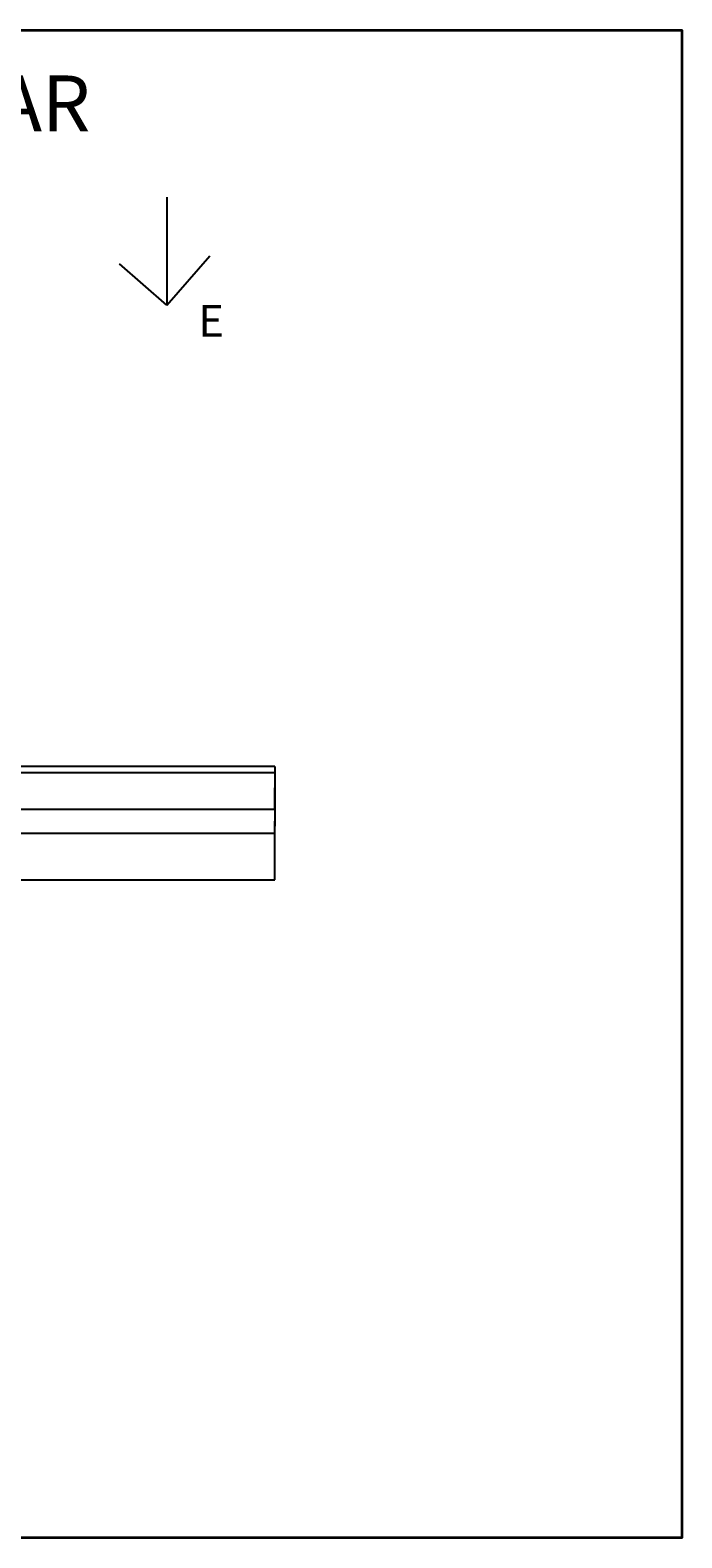
# Model space of a CAD drawing. Units: millimetres. Extents: x -5297 to 19051, y -14478 to 4427.
# Tile 4 of 4: x 10888 to 19051, y -14478 to 4427. Entities that reach past the tile are written whole.
import ezdxf

# ---------------------------------------------------------------- set-up
doc = ezdxf.new("R2010")
doc.units = ezdxf.units.MM
for name, color, linetype, lineweight in [('A-ANNO-DIMS', 2, 'Continuous', 18), ('A-ANNO-SYMB', 7, 'Continuous', 25), ('A-ANNO-TTLB', 7, 'Continuous', 35)]:
    doc.layers.add(name, color=color, linetype=linetype, lineweight=lineweight)
doc.styles.get("Standard").update_dxf_attribs({"font": 'arial.ttf'})
doc.dimstyles.get("Standard").update_dxf_attribs({"dimtxt": 0.18, "dimasz": 0.18, "dimexe": 0.18, "dimexo": 0.0625, "dimgap": 0.09, "dimtad": 0, "dimtih": 1, "dimtoh": 1, "dimdec": 4, "dimzin": 0, "dimdsep": 46, "dimtxsty": 'Standard', "dimcen": 0.09, "dimadec": 0, "dimazin": 0, "dimtfac": 1, "dimtdec": 4, "dimtofl": 0, "dimtmove": 0, "dimatfit": 3, "dimfxl": 1, "dimtolj": 1, "dimtzin": 0, "dimarcsym": 0})

# ---------------------------------------------------------------- blocks, each defined once
blk = doc.blocks.new('*D32')
at = {"layer": 'A-ANNO-DIMS', "color": 0, "lineweight": -2, "transparency": 16777216}
for p, q in [((8901.231442000004, -4880.010677000002), (13950.79322200001, -4880.010677000001)), ((13950.61322200001, -4880.190677000001), (13950.61322200001, -5553.628712470669)), ((13950.61322200001, -6227.430677000002), (13950.61322200001, -5553.992641529333)), ((8901.231442000004, -6227.610677000003), (13950.79322200001, -6227.610677000003))]:
    blk.add_line(p, q, dxfattribs=at)
at = {"layer": 'A-ANNO-DIMS', "color": 0, "transparency": 16777216}
for points in [[(13950.58322200001, -4880.190677000001), (13950.64322200001, -4880.190677000001), (13950.61322200001, -4880.010677000001)], [(13950.58322200001, -6227.430677000002), (13950.64322200001, -6227.430677000002), (13950.61322200001, -6227.610677000003)]]:
    blk.add_solid(points, dxfattribs=at)
at = {"layer": 'Defpoints', "color": 0, "transparency": 16777216}
for p in [(8901.168942000004, -4880.010677000002), (13950.61322200001, -4880.010677000001), (8901.168942000004, -6227.610677000003)]:
    blk.add_point(p, dxfattribs=at)
at = {"layer": 'A-ANNO-DIMS', "color": 0, "transparency": 16777216, "insert": (13950.61322200001, -5553.810677000004), "char_height": 0.18, "attachment_point": 5}
blk.add_mtext('\\A1;1347.6', dxfattribs=at)
blk = doc.blocks.new('*D41')
at = {"layer": 'A-ANNO-DIMS', "color": 0, "lineweight": -2, "transparency": 16777216}
for p, q in [((10027.964109, -5340.232109000002), (13950.79322200001, -5340.232109000001)), ((13950.61322200001, -5340.412109000001), (13950.61322200001, -5490.050144470669)), ((10027.964109, -5640.232109000002), (13950.79322200001, -5640.232109000001)), ((13950.61322200001, -5640.052109), (13950.61322200001, -5490.414073529333))]:
    blk.add_line(p, q, dxfattribs=at)
at = {"layer": 'A-ANNO-DIMS', "color": 0, "transparency": 16777216}
for points in [[(13950.58322200001, -5340.412109000001), (13950.64322200001, -5340.412109000001), (13950.61322200001, -5340.232109000001)], [(13950.58322200001, -5640.052109), (13950.64322200001, -5640.052109), (13950.61322200001, -5640.232109000001)]]:
    blk.add_solid(points, dxfattribs=at)
at = {"layer": 'Defpoints', "color": 0, "transparency": 16777216}
for p in [(10027.901609, -5340.232109000002), (10027.901609, -5640.232109000002), (13950.61322200001, -5640.232109000001)]:
    blk.add_point(p, dxfattribs=at)
at = {"layer": 'A-ANNO-DIMS', "color": 0, "transparency": 16777216, "insert": (13950.61322200001, -5490.232109000004), "char_height": 0.18, "attachment_point": 5}
blk.add_mtext('\\A1;300', dxfattribs=at)
blk = doc.blocks.new('*D42')
at = {"layer": 'A-ANNO-DIMS', "color": 0, "lineweight": -2, "transparency": 16777216}
for p, q in [((9951.764109000003, -4803.810677000002), (13950.79322200001, -4803.810677000001)), ((13950.61322200001, -4803.990677000001), (13950.61322200001, -5071.839428470669)), ((13950.61322200001, -5340.052109000001), (13950.61322200001, -5072.203357529332)), ((10027.964109, -5340.232109000002), (13950.79322200001, -5340.232109000001))]:
    blk.add_line(p, q, dxfattribs=at)
at = {"layer": 'A-ANNO-DIMS', "color": 0, "transparency": 16777216}
for points in [[(13950.58322200001, -4803.990677000001), (13950.64322200001, -4803.990677000001), (13950.61322200001, -4803.810677000001)], [(13950.58322200001, -5340.052109000001), (13950.64322200001, -5340.052109000001), (13950.61322200001, -5340.232109000001)]]:
    blk.add_solid(points, dxfattribs=at)
at = {"layer": 'Defpoints', "color": 0, "transparency": 16777216}
for p in [(9951.701609000003, -4803.810677000002), (10027.901609, -5340.232109000002), (13950.61322200001, -5340.232109000001)]:
    blk.add_point(p, dxfattribs=at)
at = {"layer": 'A-ANNO-DIMS', "color": 0, "transparency": 16777216, "insert": (13950.61322200001, -5072.021393000003), "char_height": 0.18, "attachment_point": 5}
blk.add_mtext('\\A1;536.4', dxfattribs=at)

msp = doc.modelspace()

# ---------------------------------------------------------------- linework, layer by layer
at = {"layer": 'A-ANNO-SYMB'}
for p, q in [((12598.74573511597, 2333.189927588928), (12598.74573511597, 979.4190577656973)), ((12598.74573511597, 979.4190577656973), (13138.1132217853, 1597.350577968709)), ((12598.74573511597, 979.4190577656973), (12006.24960145767, 1496.585021993542))]:
    msp.add_line(p, q, dxfattribs=at)
at = {"layer": 'A-ANNO-TTLB'}
msp.add_lwpolyline([(-5297.042779185286, 4427.149582433107), (19050.70310178573, 4427.149582433107), (19050.70310178573, -14478.12049047724), (-5297.042779185286, -14478.12049047724)], close=True, dxfattribs=at)

# ---------------------------------------------------------------- texts
at = {"layer": 'A-ANNO-SYMB', "insert": (12995.53034847346, 979.4190577656973), "char_height": 396.7846133574917, "attachment_point": 1}
msp.add_mtext_dynamic_manual_height_columns('{\\fArial|b1|i0|c0|p34;E}', width=396.7846133574917, gutter_width=826.634611161441, heights=[0], dxfattribs=at)
at = {"layer": 'A-ANNO-TTLB', "insert": (431.8611429029842, 3859.024494600358), "char_height": 700, "attachment_point": 1}
msp.add_mtext_dynamic_manual_height_columns('{\\fArial|b1|i0|c0|p34;FED BANK - KARMINAGAR}', width=12970.82879421404, gutter_width=826.634611161441, heights=[0], dxfattribs=at)

# ---------------------------------------------------------------- dimensions: what is measured, and where the dimension line sits
at = {"layer": 'A-ANNO-DIMS'}
for base, p1, p2, override, picture, middle in [((13950.61322200001, -4880.010677000001), (8901.168942, -6227.610677), (8901.168942, -4880.010677000001), {"dimdec": 1, "dimlfac": 1, "dimrnd": 0, "dimzin": 0, "dimdsep": 46, "dimlunit": 2}, '*D32', (13950.61322200001, -5553.810677000004)), ((13950.61322200001, -5340.232109000001), (9951.701609, -4803.810677000001), (10027.901609, -5340.232108999999), {"dimdec": 1, "dimlfac": 1, "dimrnd": 0, "dimzin": 0, "dimdsep": 46, "dimlunit": 2}, '*D42', (13950.61322200001, -5072.021393000003)), ((13950.61322200001, -5640.232109000001), (10027.901609, -5340.232108999999), (10027.901609, -5640.232108999999), {"dimdec": 0, "dimlfac": 1, "dimrnd": 0, "dimzin": 0, "dimdsep": 46, "dimlunit": 2}, '*D41', (13950.61322200001, -5490.232109000004))]:
    dim = msp.add_linear_dim(base=base, p1=p1, p2=p2, angle=90, dimstyle='Standard', override=override, dxfattribs=at)
    dim.commit()
    dim.dimension.update_dxf_attribs({"geometry": picture, "text_midpoint": middle})

doc.saveas('drawing.dxf')
